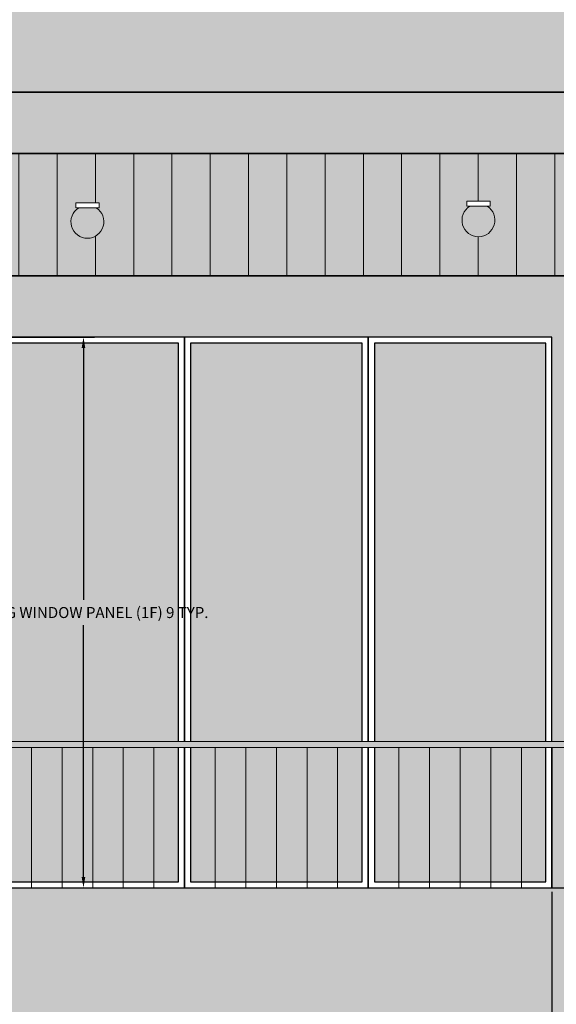
# Model space of a CAD drawing. Units: inches. Extents: x 18 to 59.8, y 2.7 to 81.2.
# Tile 5 of 9: x 35.6 to 44.4, y 29.5 to 45.6. Entities that reach past the tile are written whole.
import ezdxf

# ---------------------------------------------------------------- set-up
doc = ezdxf.new("R2010")
doc.units = ezdxf.units.IN
doc.header["$MEASUREMENT"] = 0
for name, color, linetype, lineweight in [('A-ANNO-DIMS', 2, 'Continuous', 18), ('A-ELEV', 7, 'Continuous', 35), ('A-ELEV-PATT', 8, 'Continuous', 13), ('A-ELEV-RAIL', 7, 'Continuous', 18), ('A-GLAZ', 4, 'Continuous', 25), ('E-LITE', 2, 'Continuous', 18)]:
    doc.layers.add(name, color=color, linetype=linetype, lineweight=lineweight)
doc.styles.get("Standard").update_dxf_attribs({"font": 'arial.ttf'})
doc.dimstyles.get("Standard").update_dxf_attribs({"dimtxt": 0.18, "dimasz": 0.18, "dimexe": 0.18, "dimexo": 0.0625, "dimgap": 0.09, "dimtad": 0, "dimtih": 1, "dimtoh": 1, "dimdec": 1, "dimzin": 0, "dimdsep": 46, "dimlunit": 3, "dimtxsty": 'Standard', "dimcen": 0.09, "dimadec": 0, "dimazin": 0, "dimtfac": 1, "dimtdec": 1, "dimtofl": 0, "dimtmove": 0, "dimatfit": 3, "dimfxl": 1, "dimtolj": 1, "dimtzin": 0, "dimarcsym": 0})

# ---------------------------------------------------------------- blocks, each defined once
blk = doc.blocks.new('LIGHT-CEILING-SPOT')
blk.add_lwpolyline([(0.079, 0.497), (0.459, 0.497), (0.459, 0.579), (0.079, 0.579)], close=True)
blk.add_arc((0.269, 0.269), 0.269, 122.0956, 57.9044)
blk = doc.blocks.new('WIN-SLIDING-PANEL-1F')
for points in [[(3, 2.393), (3, 9), (0, 9), (0, 2.393)], [(2.9, 2.393), (2.9, 8.9), (0.1, 8.9), (0.1, 2.393)], [(0, 2.293), (0, 0), (3, 0), (3, 2.293)], [(0.1, 2.293), (0.1, 0.1), (2.9, 0.1), (2.9, 2.293)]]:
    blk.add_lwpolyline(points)
blk = doc.blocks.new('*D8')
at = {"layer": 'A-ANNO-DIMS', "color": 0, "lineweight": -2, "transparency": 16777216}
for p, q in [((35.393, 40.441), (36.86, 40.441)), ((36.68, 40.261), (36.68, 36.149)), ((36.68, 31.621), (36.68, 35.733)), ((35.393, 31.441), (36.86, 31.441))]:
    blk.add_line(p, q, dxfattribs=at)
at = {"layer": 'A-ANNO-DIMS', "color": 0, "transparency": 16777216}
for points in [[(36.65, 40.261), (36.71, 40.261), (36.68, 40.441)], [(36.65, 31.621), (36.71, 31.621), (36.68, 31.441)]]:
    blk.add_solid(points, dxfattribs=at)
at = {"layer": 'Defpoints', "color": 0, "transparency": 16777216}
for p in [(35.33, 40.441), (36.68, 40.441), (35.33, 31.441)]:
    blk.add_point(p, dxfattribs=at)
at = {"layer": 'A-ANNO-DIMS', "color": 0, "transparency": 16777216, "insert": (36.68, 35.941), "char_height": 0.18, "attachment_point": 5}
blk.add_mtext('\\A1;SLIDING WINDOW PANEL (1F) 9 TYP.', dxfattribs=at)
blk = doc.blocks.new('*D27')
at = {"layer": 'A-ANNO-DIMS', "color": 0, "lineweight": -2, "transparency": 16777216}
for p, q in [((30.469, 31.441), (59.63, 31.441)), ((59.45, 31.261), (59.45, 30.723)), ((59.45, 29.821), (59.45, 30.359)), ((48.922, 29.641), (59.63, 29.641))]:
    blk.add_line(p, q, dxfattribs=at)
at = {"layer": 'A-ANNO-DIMS', "color": 0, "transparency": 16777216}
for points in [[(59.42, 31.261), (59.48, 31.261), (59.45, 31.441)], [(59.42, 29.821), (59.48, 29.821), (59.45, 29.641)]]:
    blk.add_solid(points, dxfattribs=at)
at = {"layer": 'Defpoints', "color": 0, "transparency": 16777216}
for p in [(30.406, 31.441), (48.86, 29.641), (59.45, 29.641)]:
    blk.add_point(p, dxfattribs=at)
at = {"layer": 'A-ANNO-DIMS', "color": 0, "transparency": 16777216, "insert": (59.45, 30.541), "char_height": 0.18, "attachment_point": 5}
blk.add_mtext('\\A1;1.8', dxfattribs=at)
blk = doc.blocks.new('*D51')
at = {"layer": 'A-ANNO-DIMS', "color": 0, "lineweight": -2, "transparency": 16777216}
for p, q in [((34.012, 44.503), (34.012, 81.211)), ((48.86, 43.503), (48.86, 81.211)), ((34.192, 81.031), (40.98, 81.031)), ((48.68, 81.031), (41.891, 81.031))]:
    blk.add_line(p, q, dxfattribs=at)
at = {"layer": 'A-ANNO-DIMS', "color": 0, "transparency": 16777216}
for points in [[(34.192, 81.061), (34.192, 81.001), (34.012, 81.031)], [(48.68, 81.061), (48.68, 81.001), (48.86, 81.031)]]:
    blk.add_solid(points, dxfattribs=at)
at = {"layer": 'Defpoints', "color": 0, "transparency": 16777216}
for p in [(48.86, 81.031), (34.012, 44.441), (48.86, 43.441)]:
    blk.add_point(p, dxfattribs=at)
at = {"layer": 'A-ANNO-DIMS', "color": 0, "transparency": 16777216, "insert": (41.436, 81.031), "char_height": 0.18, "attachment_point": 5}
blk.add_mtext('\\A1;14.848', dxfattribs=at)
blk = doc.blocks.new('*D54')
at = {"layer": 'A-ANNO-DIMS', "color": 0, "lineweight": -2, "transparency": 16777216}
for p, q in [((28.258, 33.771), (28.258, 2.671)), ((48.33, 33.352), (48.33, 2.671)), ((28.438, 2.851), (37.899, 2.851)), ((48.15, 2.851), (38.689, 2.851))]:
    blk.add_line(p, q, dxfattribs=at)
at = {"layer": 'A-ANNO-DIMS', "color": 0, "transparency": 16777216}
for points in [[(28.438, 2.881), (28.438, 2.821), (28.258, 2.851)], [(48.15, 2.881), (48.15, 2.821), (48.33, 2.851)]]:
    blk.add_solid(points, dxfattribs=at)
at = {"layer": 'Defpoints', "color": 0, "transparency": 16777216}
for p in [(28.258, 33.834), (48.33, 33.414), (48.33, 2.851)]:
    blk.add_point(p, dxfattribs=at)
at = {"layer": 'A-ANNO-DIMS', "color": 0, "transparency": 16777216, "insert": (38.294, 2.851), "char_height": 0.18, "attachment_point": 5}
blk.add_mtext('\\A1;20.07', dxfattribs=at)
blk = doc.blocks.new('*D57')
at = {"layer": 'A-ANNO-DIMS', "color": 0, "lineweight": -2, "transparency": 16777216}
for p, q in [((32.33, 31.378), (32.33, 2.671)), ((44.33, 31.378), (44.33, 2.671)), ((32.51, 2.851), (38.121, 2.851)), ((44.15, 2.851), (38.54, 2.851))]:
    blk.add_line(p, q, dxfattribs=at)
at = {"layer": 'A-ANNO-DIMS', "color": 0, "transparency": 16777216}
for points in [[(32.51, 2.881), (32.51, 2.821), (32.33, 2.851)], [(44.15, 2.881), (44.15, 2.821), (44.33, 2.851)]]:
    blk.add_solid(points, dxfattribs=at)
at = {"layer": 'Defpoints', "color": 0, "transparency": 16777216}
for p in [(32.33, 31.441), (44.33, 31.441), (44.33, 2.851)]:
    blk.add_point(p, dxfattribs=at)
at = {"layer": 'A-ANNO-DIMS', "color": 0, "transparency": 16777216, "insert": (38.33, 2.851), "char_height": 0.18, "attachment_point": 5}
blk.add_mtext('\\A1;12', dxfattribs=at)
blk = doc.blocks.new('*D58')
at = {"layer": 'A-ANNO-DIMS', "color": 0, "lineweight": -2, "transparency": 16777216}
for p, q in [((48.86, 38.622), (48.86, 2.671)), ((44.33, 31.378), (44.33, 2.671)), ((44.51, 2.851), (46.268, 2.851)), ((48.68, 2.851), (46.923, 2.851))]:
    blk.add_line(p, q, dxfattribs=at)
at = {"layer": 'A-ANNO-DIMS', "color": 0, "transparency": 16777216}
for points in [[(44.51, 2.881), (44.51, 2.821), (44.33, 2.851)], [(48.68, 2.881), (48.68, 2.821), (48.86, 2.851)]]:
    blk.add_solid(points, dxfattribs=at)
at = {"layer": 'Defpoints', "color": 0, "transparency": 16777216}
for p in [(48.86, 38.685), (44.33, 31.441), (48.86, 2.851)]:
    blk.add_point(p, dxfattribs=at)
at = {"layer": 'A-ANNO-DIMS', "color": 0, "transparency": 16777216, "insert": (46.595, 2.851), "char_height": 0.18, "attachment_point": 5}
blk.add_mtext('\\A1;4.53', dxfattribs=at)
blk = doc.blocks.new('*D61')
at = {"layer": 'A-ANNO-DIMS', "color": 0, "lineweight": -2, "transparency": 16777216}
for p, q in [((32.234, 49.378), (32.234, 2.671)), ((47.86, 49.378), (47.86, 2.671)), ((32.414, 2.851), (39.592, 2.851)), ((47.68, 2.851), (40.502, 2.851))]:
    blk.add_line(p, q, dxfattribs=at)
at = {"layer": 'A-ANNO-DIMS', "color": 0, "transparency": 16777216}
for points in [[(32.414, 2.881), (32.414, 2.821), (32.234, 2.851)], [(47.68, 2.881), (47.68, 2.821), (47.86, 2.851)]]:
    blk.add_solid(points, dxfattribs=at)
at = {"layer": 'Defpoints', "color": 0, "transparency": 16777216}
for p in [(32.234, 49.441), (47.86, 49.441), (47.86, 2.851)]:
    blk.add_point(p, dxfattribs=at)
at = {"layer": 'A-ANNO-DIMS', "color": 0, "transparency": 16777216, "insert": (40.047, 2.851), "char_height": 0.18, "attachment_point": 5}
blk.add_mtext('\\A1;15.626', dxfattribs=at)
blk = doc.blocks.new('*D66')
at = {"layer": 'A-ANNO-DIMS', "color": 0, "lineweight": -2, "transparency": 16777216}
for p, q in [((28.804, 51.378), (28.804, 2.671)), ((48.567, 51.179), (48.567, 2.671)), ((28.984, 2.851), (38.231, 2.851)), ((48.387, 2.851), (39.14, 2.851))]:
    blk.add_line(p, q, dxfattribs=at)
at = {"layer": 'A-ANNO-DIMS', "color": 0, "transparency": 16777216}
for points in [[(28.984, 2.881), (28.984, 2.821), (28.804, 2.851)], [(48.387, 2.881), (48.387, 2.821), (48.567, 2.851)]]:
    blk.add_solid(points, dxfattribs=at)
at = {"layer": 'Defpoints', "color": 0, "transparency": 16777216}
for p in [(28.804, 51.441), (48.567, 51.242), (48.567, 2.851)]:
    blk.add_point(p, dxfattribs=at)
at = {"layer": 'A-ANNO-DIMS', "color": 0, "transparency": 16777216, "insert": (38.685, 2.851), "char_height": 0.18, "attachment_point": 5}
blk.add_mtext('\\A1;19.764', dxfattribs=at)

msp = doc.modelspace()

# ---------------------------------------------------------------- hatches: boundary and pattern name
at = {"layer": 'A-ELEV-PATT'}
h = msp.add_hatch(color=256, dxfattribs=at)
h.set_gradient(color1=(255, 255, 255), color2=(199, 200, 202))
h.paths.add_polyline_path([(38.86, 75.4521, 0.4125527), (36.86, 77.4407), (21.86, 77.4407), (21.86, 22.4407), (22.86, 22.4407), (48.86, 22.4407), (48.86, 30.9234, 0.4074473), (48.3302, 31.4407), (30.4061, 31.4407, -0.7603989), (34.0116, 44.4407), (47.86, 44.4407, -0.4142136), (48.86, 43.4407), (48.86, 48.4407, 0.4142136), (47.86, 49.4407), (32.2338, 49.4407, -0.2243142), (27.8411, 52.8427, -0.8480129), (38.86, 61.4407)])
h.paths.add_polyline_path([(55.86, 77.4407), (54.86, 77.4407), (54.86, 22.2407), (55.86, 22.2407)])
h.paths.add_polyline_path([(54.86, 51.5407), (53.4401, 51.5407), (53.4401, 29.6407), (54.86, 29.6407)])
h.paths.add_polyline_path([(54.86, 61.4407), (53.4401, 57.4407), (53.4401, 51.6407), (54.86, 51.6407)])
h.paths.add_polyline_path([(54.86, 29.4407), (54.471, 29.4407), (54.471, 22.2407), (54.86, 22.2407)])
h.paths.add_polyline_path([(55.5745, 22.2407), (54.86, 22.2407), (54.5745, 22.2407), (53.9347, 21.7925), (54.5877, 21.5495)])
h.paths.add_polyline_path([(54.5991, 21.5452), (53.9443, 21.789), (53.9443, 18.4407), (54.5991, 18.4407)])
h.paths.add_polyline_path([(53.9443, 21.789), (53.9347, 21.7925), (53.5816, 21.5452), (53.5816, 18.4407), (53.9443, 18.4407)])
h.paths.add_polyline_path([(53.3648, 20.6928), (52.8956, 21.0646), (52.8956, 18.4407), (53.3648, 18.4407)])
h.paths.add_polyline_path([(52.8956, 21.0646), (50.5775, 19.4407), (50.5775, 18.4407), (52.8956, 18.4407)])
h.paths.add_polyline_path([(53.5816, 21.5452), (52.8956, 21.0646), (53.3648, 20.6928), (53.5816, 20.8447)])
h.paths.add_polyline_path([(26.8109, 19.4407), (24.9672, 20.8407), (24.9672, 18.4407), (26.8109, 18.4407)])
h.paths.add_polyline_path([(24.9672, 20.8407), (24.4165, 20.8427), (24.4165, 18.4407), (24.9672, 18.4407)])
h.paths.add_polyline_path([(24.4165, 20.8427), (24.4165, 21.2589), (24.0588, 21.5305), (24.0301, 21.5183), (24.0301, 18.4407), (24.4165, 18.4407)])
h.paths.add_polyline_path([(24.0301, 21.5183), (23.4165, 21.2589), (23.4165, 18.4407), (24.0301, 18.4407)])
h.paths.add_polyline_path([(24.0301, 21.5183), (24.0588, 21.5305), (23.1234, 22.2407), (22.1234, 22.2407), (23.4165, 21.2589)])
h.paths.add_polyline_path([(24.4165, 21.2589), (24.4165, 20.8427), (24.9672, 20.8407)])
h.paths.add_polyline_path([(47.86, 18.4407), (29.86, 18.4407), (29.86, 6.4407), (30.86, 6.4407), (30.86, 17.4407), (38.86, 17.4407), (46.86, 17.4407), (46.86, 6.4407), (47.86, 6.4407)])
h.paths.add_polyline_path([(54.5756, 15.215), (54.5756, 6.4407), (55.86, 6.4407), (55.86, 18.4407), (47.86, 18.4407), (47.86, 6.4407), (49.1482, 6.4407), (49.1482, 15.215, -1)])
h = msp.add_hatch(color=256, dxfattribs=at)
h.paths.add_polyline_path([(27.8411, 52.8427, -0.7443789), (36.86, 61.4407), (38.86, 61.4407, 0.8480129)])
h.paths.add_polyline_path([(47.86, 44.4407), (34.0116, 44.4407, 0.7603989), (30.4061, 31.4407, -0.7376246), (34.0116, 43.4407), (47.86, 43.4407, -0.4142136), (48.86, 42.4407), (48.86, 43.4407, 0.4142136)])
h.paths.add_polyline_path([(54.5756, 15.215), (54.5756, 6.4407), (55.86, 6.4407), (55.86, 18.4407), (47.86, 18.4407), (47.86, 6.4407), (49.1482, 6.4407), (49.1482, 15.215, -1)])
h.paths.add_polyline_path([(47.86, 18.4407), (29.86, 18.4407), (29.86, 6.4407), (30.86, 6.4407), (30.86, 17.4407), (38.86, 17.4407), (46.86, 17.4407), (46.86, 6.4407), (47.86, 6.4407)])
h.paths.add_polyline_path([(55.86, 77.4407), (54.86, 77.4407), (54.86, 22.2407), (55.86, 22.2407)])
h = msp.add_hatch(color=256, dxfattribs=at)
h.dxf.hatch_style = 1
h.paths.add_polyline_path([(54.86, 69.4407), (38.86, 69.4407), (38.86, 61.4407), (54.86, 61.4407)])
h.paths.add_polyline_path([(54.86, 61.4407), (38.86, 61.4407), (36.86, 61.4407, 0.443414), (27.6986, 58.4407), (48.86, 58.4407), (48.86, 57.4407), (53.4401, 57.4407)])
h.paths.add_polyline_path([(37.4994, 59.9399), (37.4994, 59.8198, -2.4106499), (37.1187, 59.8198), (37.1187, 59.9399)], flags=16)
h.paths.add_polyline_path([(42.6125, 59.8012), (42.6125, 59.9213), (42.9933, 59.9213), (42.9933, 59.8012, -2.4106499)], flags=16)
h.paths.add_polyline_path([(49.5965, 59.971), (49.5965, 60.091), (49.9773, 60.091), (49.9773, 59.971, -2.4106499)], flags=16)
h.paths.add_polyline_path([(44.4671, 57.0407), (32.6671, 57.0407), (32.6671, 56.0407), (44.4671, 56.0407)])
h.paths.add_polyline_path([(47.86, 43.4407), (46.86, 43.4407), (34.0116, 43.4407, 0.2012983), (29.3481, 41.4407), (47.86, 41.4407, 1)])
h.paths.add_polyline_path([(36.5542, 42.5145), (36.5542, 42.6346), (36.9349, 42.6346), (36.9349, 42.5145, -2.4106499)], flags=16)
h.paths.add_polyline_path([(42.939, 42.5402), (42.939, 42.6603), (43.3198, 42.6603), (43.3198, 42.5402, -2.4106499)], flags=16)
h.paths.add_polyline_path([(54.471, 29.4407), (48.86, 29.4407), (48.86, 22.2407), (54.471, 22.2407)])
h.paths.add_polyline_path([(54.5745, 22.2407), (23.1234, 22.2407), (26.8109, 19.4407), (50.5775, 19.4407)])
h.paths.add_polyline_path([(54.5756, 15.215, 1), (49.1482, 15.215), (49.1482, 6.4407), (54.5756, 6.4407)])
h.paths.add_polyline_path([(49.8323, 12.602), (49.8323, 9.1225), (49.6657, 9.1225), (49.6657, 12.602)], flags=16)
h = msp.add_hatch(dxfattribs=at)
h.set_pattern_fill('ANSI31', color=256, scale=5, angle=45, style=0)
h.paths.add_polyline_path([(54.86, 69.4407), (38.86, 69.4407), (38.86, 61.4407), (54.86, 61.4407)])
h.paths.add_polyline_path([(54.86, 61.4407), (38.86, 61.4407), (36.86, 61.4407, 0.443414), (27.6986, 58.4407), (48.86, 58.4407), (48.86, 57.4407), (53.4401, 57.4407)])
h.paths.add_polyline_path([(37.1661, 59.8577), (37.1187, 59.8577), (37.1187, 59.9399), (37.4994, 59.9399), (37.4994, 59.8577), (37.452, 59.8577, -3.476462)], flags=16)
h.paths.add_polyline_path([(42.66, 59.8391), (42.6125, 59.8391), (42.6125, 59.9213), (42.9933, 59.9213), (42.9933, 59.8391), (42.9458, 59.8391, -3.476462)], flags=16)
h.paths.add_polyline_path([(49.644, 60.0088), (49.5965, 60.0088), (49.5965, 60.091), (49.9773, 60.091), (49.9773, 60.0088), (49.9298, 60.0088, -3.476462)], flags=16)
h.paths.add_polyline_path([(44.4671, 57.0407), (32.6671, 57.0407), (32.6671, 56.0407), (44.4671, 56.0407)])
h.paths.add_polyline_path([(47.86, 43.4407), (46.86, 43.4407), (34.0116, 43.4407, 0.2012983), (29.3481, 41.4407), (47.86, 41.4407, 1)])
h.paths.add_polyline_path([(36.6016, 42.5524), (36.5542, 42.5524), (36.5542, 42.6346), (36.9349, 42.6346), (36.9349, 42.5524), (36.8875, 42.5524, -3.476462)], flags=16)
h.paths.add_polyline_path([(42.9865, 42.578), (42.939, 42.578), (42.939, 42.6603), (43.3198, 42.6603), (43.3198, 42.578), (43.2723, 42.578, -3.476462)], flags=16)
h.paths.add_polyline_path([(54.471, 29.4407), (48.86, 29.4407), (48.86, 22.2407), (54.471, 22.2407)])
h.paths.add_polyline_path([(54.5745, 22.2407), (23.1234, 22.2407), (26.8109, 19.4407), (50.5775, 19.4407)])
h.paths.add_polyline_path([(54.5756, 15.215, 1), (49.1482, 15.215), (49.1482, 6.4407), (54.5756, 6.4407)])
h.paths.add_polyline_path([(49.8323, 9.1225), (49.6657, 9.1225), (49.6657, 12.602), (49.8323, 12.602)], flags=16)
h = msp.add_hatch(color=256, dxfattribs=at)
h.paths.add_polyline_path([(36.8875, 42.5524), (36.6016, 42.5524, 3.476462)])
h.paths.add_polyline_path([(43.2723, 42.578), (42.9865, 42.578, 3.476462)])
h.paths.add_polyline_path([(37.452, 59.8577), (37.1661, 59.8577, 3.476462)])
h.paths.add_polyline_path([(42.9458, 59.8391), (42.66, 59.8391, 3.476462)])
h.paths.add_polyline_path([(49.9298, 60.0088), (49.644, 60.0088, 3.476462)])
edge = h.paths.add_edge_path()
edge.add_ellipse((29.0313, 21.3107), major_axis=(-0.2068, 0), ratio=0.411448, start_angle=0, end_angle=360)
edge = h.paths.add_edge_path()
edge.add_ellipse((32.5919, 20.2963), major_axis=(-0.2068, 0), ratio=0.411448, start_angle=0, end_angle=360)
edge = h.paths.add_edge_path()
edge.add_ellipse((35.5044, 21.3908), major_axis=(-0.2068, 0), ratio=0.411448, start_angle=0, end_angle=360)
edge = h.paths.add_edge_path()
edge.add_ellipse((39.3877, 20.1968), major_axis=(-0.2068, 0), ratio=0.411448, start_angle=0, end_angle=360)
edge = h.paths.add_edge_path()
edge.add_ellipse((43.271, 21.3659), major_axis=(-0.2068, 0), ratio=0.411448, start_angle=0, end_angle=360)
edge = h.paths.add_edge_path()
edge.add_ellipse((47.3535, 20.1471), major_axis=(-0.2068, 0), ratio=0.411448, start_angle=0, end_angle=360)
at = {"layer": 'A-ELEV-PATT', "transparency": 33554620}
h = msp.add_hatch(color=256, dxfattribs=at)
h.set_gradient(color1=(147, 149, 152))
edge = h.paths.add_edge_path()
edge.add_line((32.5671, 55.9407), (32.5671, 57.1407))
edge.add_line((32.5671, 57.1407), (44.5671, 57.1407))
edge.add_line((44.5671, 57.1407), (44.5671, 55.9407))
edge.add_line((44.5671, 55.9407), (44.5671, 51.5407))
edge.add_line((44.5671, 51.5407), (47.9208, 51.5407))
edge.add_spline(control_points=[(47.9208, 51.5407), (48.1524, 51.5145), (48.3597, 51.3781), (48.5671, 51.2416)], knot_values=[0, 0, 0, 0, 0.7121901, 0.7121901, 0.7121901, 0.7121901], degree=3, periodic=0)
edge.add_line((48.5671, 51.2416), (48.5671, 49.1479))
edge.add_arc((47.86, 48.4407), 1, 5.73917, 45, ccw=False)
edge.add_line((48.855, 48.5407), (48.86, 48.5407))
edge.add_line((48.86, 48.5407), (48.86, 49.4407))
edge.add_line((48.86, 49.4407), (48.86, 58.4407))
edge.add_line((48.86, 58.4407), (27.6986, 58.4407))
edge.add_arc((33.6382, 55.7911), 6.5038, 155.95802, 220.80748)
edge.add_line((28.7154, 51.5407), (32.5671, 51.5407))
edge.add_line((32.5671, 51.5407), (32.5671, 55.9407))
edge = h.paths.add_edge_path()
edge.add_line((32.3302, 40.4407), (35.3302, 40.4407))
edge.add_line((35.3302, 40.4407), (38.3302, 40.4407))
edge.add_line((38.3302, 40.4407), (41.3302, 40.4407))
edge.add_line((41.3302, 40.4407), (44.3302, 40.4407))
edge.add_line((44.3302, 40.4407), (44.3302, 33.8336))
edge.add_line((44.3302, 33.8336), (47.6839, 33.8336))
edge.add_spline(control_points=[(47.6839, 33.8336), (47.9155, 33.8074), (48.1229, 33.671), (48.3302, 33.5345)], knot_values=[0, 0, 0, 0, 0.7121901, 0.7121901, 0.7121901, 0.7121901], degree=3, periodic=0)
edge.add_line((48.3302, 33.5345), (48.3302, 31.4407))
edge.add_arc((48.3304, 30.911), 0.5297, 1.3425, 90.01573, ccw=False)
edge.add_line((48.86, 30.9234), (48.86, 38.6846))
edge.add_line((48.86, 38.6846), (50.793, 38.6846))
edge.add_line((50.793, 38.6846), (50.793, 41.316))
edge.add_line((50.793, 41.316), (52.927, 41.316))
edge.add_line((52.927, 41.316), (52.927, 38.6846))
edge.add_line((52.927, 38.6846), (53.4401, 38.6846))
edge.add_line((53.4401, 38.6846), (53.4401, 48.4407))
edge.add_line((53.4401, 48.4407), (48.86, 48.4407))
edge.add_line((48.86, 48.4407), (48.86, 42.4407))
edge.add_arc((47.86, 42.4407), 1, -90, 0, ccw=False)
edge.add_line((47.86, 41.4407), (29.3481, 41.4407))
edge.add_arc((34.0631, 36.8836), 6.5573, 135.97541, 207.71831)
edge.add_line((28.2583, 33.8336), (32.3302, 33.8336))
edge.add_line((32.3302, 33.8336), (32.3302, 40.4407))
h.paths.add_polyline_path([(53.4401, 57.4407), (48.86, 57.4407), (48.86, 51.6407), (53.4401, 51.6407)])
h.paths.add_polyline_path([(29.5671, 51.4407), (28.8035, 51.4407, 0.040451), (29.5671, 50.7191)], flags=17)
h.paths.add_polyline_path([(30.0671, 51.4407), (29.5671, 51.4407), (29.5671, 50.7191, 0.0237787), (30.0671, 50.3554)], flags=17)
h.paths.add_polyline_path([(30.5671, 51.4407), (30.0671, 51.4407), (30.0671, 50.3554, 0.0223729), (30.5671, 50.0581)], flags=17)
h.paths.add_polyline_path([(31.0671, 51.4407), (30.5671, 51.4407), (30.5671, 50.0581, 0.021345), (31.0671, 49.8171)], flags=17)
h.paths.add_polyline_path([(31.5671, 51.4407), (31.0671, 51.4407), (31.0671, 49.8171, 0.0205858), (31.5671, 49.6259)], flags=17)
h.paths.add_polyline_path([(32.0671, 51.4407), (31.5671, 51.4407), (31.5671, 49.6259, 0.0200299), (32.0671, 49.4799)], flags=17)
h.paths.add_polyline_path([(32.5671, 51.4407), (32.0671, 51.4407), (32.0671, 49.4799, 0.0065845), (32.2338, 49.4407), (32.5671, 49.4407)], flags=17)
h.paths.add_polyline_path([(45.0671, 51.4407), (44.5671, 51.4407), (44.5671, 49.4407), (45.0671, 49.4407)], flags=17)
h.paths.add_polyline_path([(45.5671, 51.4407), (45.0671, 51.4407), (45.0671, 49.4407), (45.5671, 49.4407)], flags=17)
h.paths.add_polyline_path([(46.0671, 51.4407), (45.5671, 51.4407), (45.5671, 49.4407), (46.0671, 49.4407)], flags=17)
h.paths.add_polyline_path([(46.5671, 51.4407), (46.0671, 51.4407), (46.0671, 49.4407), (46.5671, 49.4407)], flags=17)
h.paths.add_polyline_path([(47.0671, 51.4407), (46.5671, 51.4407), (46.5671, 49.4407), (47.0671, 49.4407)], flags=17)
h.paths.add_polyline_path([(47.5671, 51.4407), (47.0671, 51.4407), (47.0671, 49.4407), (47.5671, 49.4407)], flags=17)
edge = h.paths.add_edge_path(flags=17)
edge.add_spline(control_points=[(48.0671, 51.4184), (48.0217, 51.4311), (47.9752, 51.4389), (47.9273, 51.4407)], knot_values=[0.570104, 0.570104, 0.570104, 0.570104, 0.7151116, 0.7151116, 0.7151116, 0.7151116], degree=3, periodic=0)
edge.add_line((47.9273, 51.4407), (47.5671, 51.4407))
edge.add_line((47.5671, 51.4407), (47.5671, 49.4407))
edge.add_line((47.5671, 49.4407), (47.86, 49.4407))
edge.add_arc((47.86, 48.4407), 1, 78.04714, 90, ccw=False)
edge.add_line((48.0671, 49.4191), (48.0671, 51.4184))
edge = h.paths.add_edge_path(flags=17)
edge.add_spline(control_points=[(48.5671, 51.1212), (48.4062, 51.2449), (48.2454, 51.3687), (48.0671, 51.4184)], knot_values=[0, 0, 0, 0, 0.570104, 0.570104, 0.570104, 0.570104], degree=3, periodic=0)
edge.add_line((48.0671, 51.4184), (48.0671, 49.4191))
edge.add_arc((47.86, 48.4407), 1, 45, 78.04714, ccw=False)
edge.add_line((48.5671, 49.1479), (48.5671, 51.1212))
h.paths.add_polyline_path([(49.36, 51.5407), (48.86, 51.5407), (48.86, 49.4407), (48.86, 48.5407), (49.36, 48.5407)])
h.paths.add_polyline_path([(49.86, 51.5407), (49.36, 51.5407), (49.36, 48.5407), (49.86, 48.5407)])
h.paths.add_polyline_path([(50.36, 51.5407), (49.86, 51.5407), (49.86, 48.5407), (50.36, 48.5407)])
h.paths.add_polyline_path([(50.86, 51.5407), (50.36, 51.5407), (50.36, 48.5407), (50.86, 48.5407)])
h.paths.add_polyline_path([(51.36, 51.5407), (50.86, 51.5407), (50.86, 48.5407), (51.36, 48.5407)])
h.paths.add_polyline_path([(51.86, 51.5407), (51.36, 51.5407), (51.36, 48.5407), (51.86, 48.5407)])
h.paths.add_polyline_path([(52.36, 51.5407), (51.86, 51.5407), (51.86, 48.5407), (52.36, 48.5407)])
h.paths.add_polyline_path([(52.86, 51.5407), (52.36, 51.5407), (52.36, 48.5407), (52.86, 48.5407)])
h.paths.add_polyline_path([(53.36, 51.5407), (52.86, 51.5407), (52.86, 48.5407), (53.36, 48.5407)])
h.paths.add_polyline_path([(53.4401, 38.6846), (48.86, 38.6846), (48.86, 30.9234), (48.86, 29.6407), (53.4401, 29.6407)])
h.paths.add_polyline_path([(28.8302, 33.7336), (28.3119, 33.7336, 0.0364452), (28.8302, 32.9319)], flags=17)
h.paths.add_polyline_path([(29.3302, 33.7336), (28.8302, 33.7336), (28.8302, 32.9319, 0.0294201), (29.3302, 32.3451)], flags=17)
h.paths.add_polyline_path([(29.8302, 33.7336), (29.3302, 33.7336), (29.3302, 32.3451, 0.0261691), (29.8302, 31.8755)], flags=17)
h.paths.add_polyline_path([(30.3302, 33.7336), (29.8302, 33.7336), (29.8302, 31.8755, 0.0240263), (30.3302, 31.4925)], flags=17)
h.paths.add_polyline_path([(30.8302, 33.7336), (30.3302, 33.7336), (30.3302, 31.4925, 0.0035006), (30.4061, 31.4407), (30.8302, 31.4407)], flags=17)
h.paths.add_polyline_path([(31.3302, 33.7336), (30.8302, 33.7336), (30.8302, 31.4407), (31.3302, 31.4407)], flags=17)
h.paths.add_polyline_path([(31.8302, 33.7336), (31.3302, 33.7336), (31.3302, 31.4407), (31.8302, 31.4407)], flags=17)
h.paths.add_polyline_path([(32.3302, 33.7336), (31.8302, 33.7336), (31.8302, 31.4407), (32.3302, 31.4407)], flags=17)
h.paths.add_polyline_path([(44.8302, 33.7336), (44.3302, 33.7336), (44.3302, 31.4407), (44.8302, 31.4407)], flags=17)
h.paths.add_polyline_path([(45.3302, 33.7336), (44.8302, 33.7336), (44.8302, 31.4407), (45.3302, 31.4407)], flags=17)
h.paths.add_polyline_path([(45.8302, 33.7336), (45.3302, 33.7336), (45.3302, 31.4407), (45.8302, 31.4407)], flags=17)
h.paths.add_polyline_path([(46.3302, 33.7336), (45.8302, 33.7336), (45.8302, 31.4407), (46.3302, 31.4407)], flags=17)
h.paths.add_polyline_path([(46.8302, 33.7336), (46.3302, 33.7336), (46.3302, 31.4407), (46.8302, 31.4407)], flags=17)
h.paths.add_polyline_path([(47.3302, 33.7336), (46.8302, 33.7336), (46.8302, 31.4407), (47.3302, 31.4407)], flags=17)
edge = h.paths.add_edge_path(flags=16)
edge.add_spline(control_points=[(47.8302, 33.7113), (47.7849, 33.7239), (47.7384, 33.7318), (47.6905, 33.7336)], knot_values=[0.570104, 0.570104, 0.570104, 0.570104, 0.7151116, 0.7151116, 0.7151116, 0.7151116], degree=3, periodic=0)
edge.add_line((47.6905, 33.7336), (47.3302, 33.7336))
edge.add_line((47.3302, 33.7336), (47.3302, 31.4407))
edge.add_line((47.3302, 31.4407), (47.8302, 31.4407))
edge.add_line((47.8302, 31.4407), (47.8302, 33.7113))
h.paths.add_polyline_path([(48.86, 38.6846), (50.793, 38.6846), (50.793, 41.316), (52.927, 41.316), (52.927, 38.6846), (53.4401, 38.6846), (53.4401, 48.4407), (48.86, 48.4407), (48.86, 42.4407, -0.4142136), (47.86, 41.4407), (29.3481, 41.4407, 0.3236799), (28.2583, 33.8336), (32.3302, 33.8336), (32.3302, 40.4407), (35.3302, 40.4407), (38.3302, 40.4407), (41.3302, 40.4407), (44.3302, 40.4407), (44.3302, 33.8336), (28.2583, 33.8336, 0.0043267), (28.3119, 33.7336), (28.8302, 33.7336), (29.3302, 33.7336), (29.8302, 33.7336), (30.3302, 33.7336), (30.8302, 33.7336), (31.3302, 33.7336), (31.8302, 33.7336), (32.3302, 33.7336), (47.3302, 33.7336), (47.3302, 31.4407), (47.8302, 31.4407), (48.3302, 31.4407, -0.4074473), (48.86, 30.9234)])
edge = h.paths.add_edge_path(flags=0)
edge.add_spline(control_points=[(47.8302, 33.7113), (47.7849, 33.7239), (47.7384, 33.7318), (47.6905, 33.7336)], knot_values=[0.570104, 0.570104, 0.570104, 0.570104, 0.7151116, 0.7151116, 0.7151116, 0.7151116], degree=3, periodic=0)
edge.add_line((47.6905, 33.7336), (47.3302, 33.7336))
edge.add_line((47.3302, 33.7336), (47.3302, 31.4407))
edge.add_line((47.3302, 31.4407), (47.8302, 31.4407))
edge.add_line((47.8302, 31.4407), (47.8302, 33.7113))
h = msp.add_hatch(color=256, dxfattribs=at)
h.set_gradient(color1=(147, 149, 152))
edge = h.paths.add_edge_path()
edge.add_line((44.3302, 33.8336), (47.6839, 33.8336))
edge.add_spline(control_points=[(47.6839, 33.8336), (47.9155, 33.8074), (48.1229, 33.671), (48.3302, 33.5345)], knot_values=[0, 0, 0, 0, 0.7121901, 0.7121901, 0.7121901, 0.7121901], degree=3, periodic=0)
edge.add_line((48.3302, 33.5345), (48.3302, 31.4407))
edge.add_arc((48.3304, 30.911), 0.5297, 1.3425, 90.01573, ccw=False)
edge.add_line((48.86, 30.9234), (48.86, 38.6846))
edge.add_line((48.86, 38.6846), (50.793, 38.6846))
edge.add_line((50.793, 38.6846), (50.793, 41.316))
edge.add_line((50.793, 41.316), (52.927, 41.316))
edge.add_line((52.927, 41.316), (52.927, 38.6846))
edge.add_line((52.927, 38.6846), (53.4401, 38.6846))
edge.add_line((53.4401, 38.6846), (53.4401, 48.4407))
edge.add_line((53.4401, 48.4407), (48.86, 48.4407))
edge.add_line((48.86, 48.4407), (48.86, 42.4407))
edge.add_arc((47.86, 42.4407), 1, -90, 0, ccw=False)
edge.add_line((47.86, 41.4407), (29.3481, 41.4407))
edge.add_arc((34.0631, 36.8836), 6.5573, 135.97541, 207.71831)
edge.add_line((28.2583, 33.8336), (32.3302, 33.8336))
edge.add_line((32.3302, 33.8336), (32.3302, 40.4407))
edge.add_line((32.3302, 40.4407), (35.3302, 40.4407))
edge.add_line((35.3302, 40.4407), (38.3302, 40.4407))
edge.add_line((38.3302, 40.4407), (41.3302, 40.4407))
edge.add_line((41.3302, 40.4407), (44.3302, 40.4407))
edge.add_line((44.3302, 40.4407), (44.3302, 33.8336))
h = msp.add_hatch(color=256, dxfattribs=at)
h.set_gradient(color1=(173, 221, 247))
h.paths.add_polyline_path([(35.2302, 40.3407), (32.4302, 40.3407), (32.4302, 33.8336), (35.2302, 33.8336)])
h.paths.add_polyline_path([(32.8302, 33.7336), (32.4302, 33.7336), (32.4302, 31.5407), (32.8302, 31.5407)])
h.paths.add_polyline_path([(33.3302, 33.7336), (32.8302, 33.7336), (32.8302, 31.5407), (33.3302, 31.5407)])
h.paths.add_polyline_path([(33.8302, 33.7336), (33.3302, 33.7336), (33.3302, 31.5407), (33.8302, 31.5407)])
h.paths.add_polyline_path([(34.3302, 33.7336), (33.8302, 33.7336), (33.8302, 31.5407), (34.3302, 31.5407)])
h.paths.add_polyline_path([(34.8302, 33.7336), (34.3302, 33.7336), (34.3302, 31.5407), (34.8302, 31.5407)])
h.paths.add_polyline_path([(35.2302, 33.7336), (34.8302, 33.7336), (34.8302, 31.5407), (35.2302, 31.5407)])
h.paths.add_polyline_path([(38.2302, 40.3407), (35.4302, 40.3407), (35.4302, 33.8336), (38.2302, 33.8336)])
h.paths.add_polyline_path([(35.8302, 33.7336), (35.4302, 33.7336), (35.4302, 31.5407), (35.8302, 31.5407)])
h.paths.add_polyline_path([(36.3302, 33.7336), (35.8302, 33.7336), (35.8302, 31.5407), (36.3302, 31.5407)])
h.paths.add_polyline_path([(36.8302, 33.7336), (36.3302, 33.7336), (36.3302, 31.5407), (36.8302, 31.5407)])
h.paths.add_polyline_path([(37.3302, 33.7336), (36.8302, 33.7336), (36.8302, 31.5407), (37.3302, 31.5407)])
h.paths.add_polyline_path([(37.8302, 33.7336), (37.3302, 33.7336), (37.3302, 31.5407), (37.8302, 31.5407)])
h.paths.add_polyline_path([(38.2302, 33.7336), (37.8302, 33.7336), (37.8302, 31.5407), (38.2302, 31.5407)])
h.paths.add_polyline_path([(41.2302, 40.3407), (38.4302, 40.3407), (38.4302, 33.8336), (41.2302, 33.8336)])
h.paths.add_polyline_path([(44.2302, 40.3407), (41.4302, 40.3407), (41.4302, 33.8336), (44.2302, 33.8336)])
h.paths.add_polyline_path([(38.8302, 33.7336), (38.4302, 33.7336), (38.4302, 31.5407), (38.8302, 31.5407)])
h.paths.add_polyline_path([(39.3302, 33.7336), (38.8302, 33.7336), (38.8302, 31.5407), (39.3302, 31.5407)])
h.paths.add_polyline_path([(39.8302, 33.7336), (39.3302, 33.7336), (39.3302, 31.5407), (39.8302, 31.5407)])
h.paths.add_polyline_path([(40.3302, 33.7336), (39.8302, 33.7336), (39.8302, 31.5407), (40.3302, 31.5407)])
h.paths.add_polyline_path([(40.8302, 33.7336), (40.3302, 33.7336), (40.3302, 31.5407), (40.8302, 31.5407)])
h.paths.add_polyline_path([(41.2302, 33.7336), (40.8302, 33.7336), (40.8302, 31.5407), (41.2302, 31.5407)])
h.paths.add_polyline_path([(41.8302, 33.7336), (41.4302, 33.7336), (41.4302, 31.5407), (41.8302, 31.5407)])
h.paths.add_polyline_path([(42.3302, 33.7336), (41.8302, 33.7336), (41.8302, 31.5407), (42.3302, 31.5407)])
h.paths.add_polyline_path([(42.8302, 33.7336), (42.3302, 33.7336), (42.3302, 31.5407), (42.8302, 31.5407)])
h.paths.add_polyline_path([(43.3302, 33.7336), (42.8302, 33.7336), (42.8302, 31.5407), (43.3302, 31.5407)])
h.paths.add_polyline_path([(43.8302, 33.7336), (43.3302, 33.7336), (43.3302, 31.5407), (43.8302, 31.5407)])
h.paths.add_polyline_path([(44.2302, 33.7336), (43.8302, 33.7336), (43.8302, 31.5407), (44.2302, 31.5407)])
at = {"layer": 'A-ELEV-PATT'}
h = msp.add_hatch(color=256, dxfattribs=at)
h.paths.add_polyline_path([(38.86, 17.4407), (30.86, 17.4407), (30.86, 6.4407), (30.96, 6.4407), (30.96, 17.3407), (38.86, 17.3407)])
h.paths.add_polyline_path([(46.86, 17.4407), (38.86, 17.4407), (38.86, 17.3407), (46.76, 17.3407), (46.76, 6.4407), (46.86, 6.4407)])
h.paths.add_polyline_path([(49.8323, 12.602), (49.6657, 12.602), (49.6657, 9.1225), (49.8323, 9.1225)])
h.paths.add_polyline_path([(48.86, 22.4407), (21.86, 22.4407), (21.86, 22.2407), (48.86, 22.2407)])
h.paths.add_polyline_path([(54.86, 29.6407), (48.86, 29.6407), (48.86, 29.4407), (54.86, 29.4407)])
edge = h.paths.add_edge_path()
edge.add_spline(control_points=[(48.3302, 33.5345), (48.1229, 33.671), (47.9155, 33.8074), (47.6839, 33.8336)], knot_values=[0, 0, 0, 0, 0.7121901, 0.7121901, 0.7121901, 0.7121901], degree=3, periodic=0)
edge.add_line((47.6839, 33.8336), (28.2583, 33.8336))
edge.add_arc((34.0631, 36.8836), 6.5573, 207.71831, 208.7099)
edge.add_line((28.3119, 33.7336), (47.6238, 33.7336))
edge.add_spline(control_points=[(47.6238, 33.7336), (47.6461, 33.7341), (47.6685, 33.7345), (47.6905, 33.7336)], knot_values=[0, 0, 0, 0, 0.0667446, 0.0667446, 0.0667446, 0.0667446], degree=3, periodic=0)
edge.add_spline(control_points=[(47.6905, 33.7336), (47.7384, 33.7318), (47.7849, 33.7239), (47.8302, 33.7113)], knot_values=[0.570104, 0.570104, 0.570104, 0.570104, 0.7151116, 0.7151116, 0.7151116, 0.7151116], degree=3, periodic=0)
edge.add_spline(control_points=[(47.8302, 33.7113), (48.0085, 33.6616), (48.1694, 33.5378), (48.3302, 33.4141)], knot_values=[0, 0, 0, 0, 0.570104, 0.570104, 0.570104, 0.570104], degree=3, periodic=0)
edge.add_line((48.3302, 33.4141), (48.3302, 33.5345))
h = msp.add_hatch(color=256, dxfattribs=at)
edge = h.paths.add_edge_path()
edge.add_spline(control_points=[(48.3302, 33.5345), (48.1229, 33.671), (47.9155, 33.8074), (47.6839, 33.8336)], knot_values=[0, 0, 0, 0, 0.7121901, 0.7121901, 0.7121901, 0.7121901], degree=3, periodic=0)
edge.add_line((47.6839, 33.8336), (28.2583, 33.8336))
edge.add_arc((34.0631, 36.8836), 6.5573, 207.71831, 208.7099)
edge.add_line((28.3119, 33.7336), (47.6238, 33.7336))
edge.add_spline(control_points=[(47.6238, 33.7336), (47.6461, 33.7341), (47.6685, 33.7345), (47.6905, 33.7336)], knot_values=[0, 0, 0, 0, 0.0667446, 0.0667446, 0.0667446, 0.0667446], degree=3, periodic=0)
edge.add_spline(control_points=[(47.6905, 33.7336), (47.7384, 33.7318), (47.7849, 33.7239), (47.8302, 33.7113)], knot_values=[0.570104, 0.570104, 0.570104, 0.570104, 0.7151116, 0.7151116, 0.7151116, 0.7151116], degree=3, periodic=0)
edge.add_spline(control_points=[(47.8302, 33.7113), (48.0085, 33.6616), (48.1694, 33.5378), (48.3302, 33.4141)], knot_values=[0, 0, 0, 0, 0.570104, 0.570104, 0.570104, 0.570104], degree=3, periodic=0)
edge.add_line((48.3302, 33.4141), (48.3302, 33.5345))

# ---------------------------------------------------------------- linework, layer by layer
at = {"layer": 'A-ELEV'}
for p, q in [((47.86, 44.4407), (34.0116, 44.4407)), ((47.86, 43.4407), (34.0116, 43.4407)), ((47.86, 41.4407), (29.3481, 41.4407))]:
    msp.add_line(p, q, dxfattribs=at)
at = {"layer": 'A-ELEV-RAIL'}
for p, q in [((47.6839, 33.8336), (28.2583, 33.8336)), ((47.6905, 33.7336), (28.3119, 33.7336)), ((35.8302, 31.4407), (35.8302, 33.7336)), ((36.3302, 31.4407), (36.3302, 33.7336)), ((36.8302, 31.4407), (36.8302, 33.7336)), ((37.3302, 31.4407), (37.3302, 33.7336)), ((37.8302, 31.4407), (37.8302, 33.7336)), ((38.3302, 31.4407), (38.3302, 33.7336)), ((38.8302, 31.4407), (38.8302, 33.7336)), ((39.3302, 31.4407), (39.3302, 33.7336)), ((39.8302, 31.4407), (39.8302, 33.7336)), ((40.3302, 31.4407), (40.3302, 33.7336)), ((40.8302, 31.4407), (40.8302, 33.7336)), ((41.3302, 31.4407), (41.3302, 33.7336)), ((41.8302, 31.4407), (41.8302, 33.7336)), ((42.3302, 31.4407), (42.3302, 33.7336)), ((42.8302, 31.4407), (42.8302, 33.7336)), ((43.3302, 31.4407), (43.3302, 33.7336)), ((43.8302, 31.4407), (43.8302, 33.7336)), ((44.3302, 31.4407), (44.3302, 33.7336)), ((48.3305, 31.4407), (30.4061, 31.4407))]:
    msp.add_line(p, q, dxfattribs=at)

# ---------------------------------------------------------------- block references
at = {"layer": 'A-GLAZ'}
for p in [(35.33, 31.441), (38.33, 31.441), (41.33, 31.441)]:
    msp.add_blockref('WIN-SLIDING-PANEL-1F', p, dxfattribs=at)
at = {"layer": 'E-LITE'}
for p in [(36.4755, 42.0557), (42.8603, 42.0813)]:
    msp.add_blockref('LIGHT-CEILING-SPOT', p, dxfattribs=at)

# ---------------------------------------------------------------- dimensions: what is measured, and where the dimension line sits
at = {"layer": 'A-ANNO-DIMS'}
for base, p1, p2, override, picture, middle in [((48.86, 81.0307), (34.0116, 44.4407), (48.86, 43.4407), {"dimdec": 3, "dimlfac": 1, "dimrnd": 0, "dimzin": 0, "dimdsep": 46, "dimlunit": 2}, '*D51', (41.4358, 81.0307)), ((48.5671, 2.8507), (28.8035, 51.4407), (48.5671, 51.2416), {"dimdec": 3, "dimlfac": 1, "dimrnd": 0, "dimzin": 0, "dimdsep": 46, "dimlunit": 2}, '*D66', (38.6853, 2.8507)), ((47.86, 2.8507), (32.2338, 49.4407), (47.86, 49.4407), {"dimdec": 3, "dimlfac": 1, "dimrnd": 0, "dimzin": 0, "dimdsep": 46, "dimlunit": 2}, '*D61', (40.0469, 2.8507)), ((48.86, 2.8507), (44.3302, 31.4407), (48.86, 38.6846), {"dimdec": 2, "dimlfac": 1, "dimrnd": 0, "dimzin": 0, "dimdsep": 46, "dimlunit": 2}, '*D58', (46.5951, 2.8507)), ((48.3302, 2.8507), (28.2583, 33.8336), (48.3302, 33.4141), {"dimdec": 2, "dimlfac": 1, "dimrnd": 0, "dimzin": 0, "dimdsep": 46, "dimlunit": 2}, '*D54', (38.2942, 2.8507)), ((44.3302, 2.8507), (32.3302, 31.4407), (44.3302, 31.4407), {"dimdec": 0, "dimlfac": 1, "dimrnd": 0, "dimzin": 0, "dimdsep": 46, "dimlunit": 2}, '*D57', (38.3302, 2.8507))]:
    dim = msp.add_linear_dim(base=base, p1=p1, p2=p2, dimstyle='Standard', override=override, dxfattribs=at)
    dim.commit()
    dim.dimension.update_dxf_attribs({"geometry": picture, "text_midpoint": middle})
dim = msp.add_linear_dim(base=(36.6802, 40.4407), p1=(35.3302, 31.4407), p2=(35.3302, 40.4407), angle=90, text='SLIDING WINDOW PANEL (1F) <> TYP.', dimstyle='Standard', override={"dimdec": 0, "dimlfac": 1, "dimrnd": 0, "dimzin": 0, "dimdsep": 46, "dimlunit": 2}, dxfattribs=at)
dim.commit()
dim.dimension.update_dxf_attribs({"geometry": '*D8', "text_midpoint": (36.6802, 35.9407)})
dim = msp.add_linear_dim(base=(59.45, 29.6407), p1=(30.4061, 31.4407), p2=(48.86, 29.6407), angle=90, dimstyle='Standard', override={"dimdec": 1, "dimlfac": 1, "dimrnd": 0, "dimzin": 0, "dimdsep": 46, "dimlunit": 2}, dxfattribs=at)
dim.commit()
dim.dimension.update_dxf_attribs({"geometry": '*D27', "text_midpoint": (59.45, 30.5407)})

doc.saveas('drawing.dxf')
